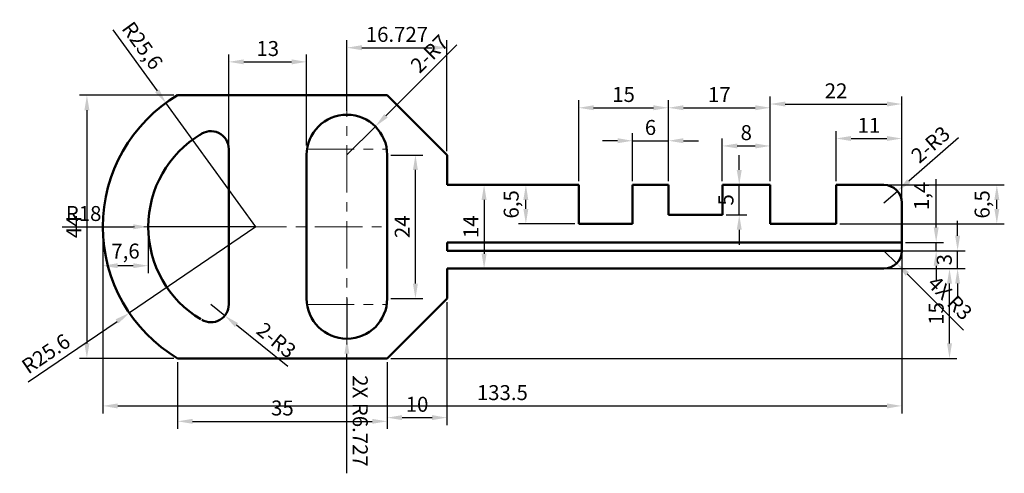
# Model space of a CAD drawing. Units: millimetres. Extents: x 2573 to 2737, y 1736 to 1812.
import ezdxf

# ---------------------------------------------------------------- set-up
doc = ezdxf.new("R2010")
doc.units = ezdxf.units.MM
doc.linetypes.add('CENTER', pattern=[50.8, 31.75, -6.35, 6.35, -6.35])
for name, color, linetype, lineweight in [('M-CNTR', 4, 'CENTER', 18), ('M-DIMS', 2, 'Continuous', 25), ('M-OUTL', 7, 'Continuous', 50)]:
    doc.layers.add(name, color=color, linetype=linetype, lineweight=lineweight)
doc.styles.get("Standard").update_dxf_attribs({"font": 'arial.ttf'})
doc.dimstyles.new('ISO-25', dxfattribs={"dimtxt": 2.5, "dimasz": 2.5, "dimexe": 1.25, "dimexo": 0.625, "dimtad": 1, "dimtxsty": 'Standard', "dimcen": 2.5, "dimadec": 0, "dimazin": 0, "dimtfac": 1, "dimtmove": 0, "dimatfit": 3, "dimfxl": 1, "dimarcsym": 0})

# ---------------------------------------------------------------- blocks, each defined once
blk = doc.blocks.new('*D1')
at = {"layer": 'Defpoints', "color": 0, "transparency": 16777216}
for p in [(2599.21, 1799.66), (2584.05, 1755.66), (2599.21, 1755.66)]:
    blk.add_point(p, dxfattribs=at)
at = {"layer": 'M-DIMS', "color": 0, "lineweight": -2, "transparency": 16777216}
for p, q in [((2598.59, 1799.66), (2582.8, 1799.66)), ((2584.05, 1797.16), (2584.05, 1758.16)), ((2598.59, 1755.66), (2582.8, 1755.66))]:
    blk.add_line(p, q, dxfattribs=at)
at = {"layer": 'M-DIMS', "color": 0, "transparency": 16777216}
for points in [[(2583.63, 1797.16), (2584.47, 1797.16), (2584.05, 1799.66)], [(2583.63, 1758.16), (2584.47, 1758.16), (2584.05, 1755.66)]]:
    blk.add_solid(points, dxfattribs=at)
at = {"layer": 'M-DIMS', "color": 0, "transparency": 16777216, "insert": (2582.17, 1777.66), "char_height": 2.5, "attachment_point": 5, "rotation": 90}
blk.add_mtext('44', dxfattribs=at)
blk = doc.blocks.new('*D2')
at = {"layer": 'Defpoints', "color": 0, "transparency": 16777216}
for p in [(2620.76, 1805.24), (2607.76, 1790.66), (2620.76, 1790.66)]:
    blk.add_point(p, dxfattribs=at)
at = {"layer": 'M-DIMS', "color": 0, "lineweight": -2, "transparency": 16777216}
for p, q in [((2607.76, 1791.28), (2607.76, 1806.49)), ((2620.76, 1791.28), (2620.76, 1806.49)), ((2610.26, 1805.24), (2618.26, 1805.24))]:
    blk.add_line(p, q, dxfattribs=at)
at = {"layer": 'M-DIMS', "color": 0, "transparency": 16777216}
for points in [[(2610.26, 1805.65), (2610.26, 1804.82), (2607.76, 1805.24)], [(2618.26, 1805.65), (2618.26, 1804.82), (2620.76, 1805.24)]]:
    blk.add_solid(points, dxfattribs=at)
at = {"layer": 'M-DIMS', "color": 0, "transparency": 16777216, "insert": (2614.26, 1807.14), "char_height": 2.5, "attachment_point": 5}
blk.add_mtext('13', dxfattribs=at)
blk = doc.blocks.new('*D3')
at = {"layer": 'Defpoints', "color": 0, "transparency": 16777216}
for p in [(2599.21, 1755.66), (2634.21, 1755.66), (2634.21, 1745.13)]:
    blk.add_point(p, dxfattribs=at)
at = {"layer": 'M-DIMS', "color": 0, "lineweight": -2, "transparency": 16777216}
for p, q in [((2599.21, 1755.04), (2599.21, 1743.88)), ((2634.21, 1755.04), (2634.21, 1743.88)), ((2601.71, 1745.13), (2631.71, 1745.13))]:
    blk.add_line(p, q, dxfattribs=at)
at = {"layer": 'M-DIMS', "color": 0, "transparency": 16777216}
for points in [[(2601.71, 1745.55), (2601.71, 1744.72), (2599.21, 1745.13)], [(2631.71, 1745.55), (2631.71, 1744.72), (2634.21, 1745.13)]]:
    blk.add_solid(points, dxfattribs=at)
at = {"layer": 'M-DIMS', "color": 0, "transparency": 16777216, "insert": (2616.71, 1747.04), "char_height": 2.5, "attachment_point": 5}
blk.add_mtext('35', dxfattribs=at)
blk = doc.blocks.new('*D4')
at = {"layer": 'Defpoints', "color": 0, "transparency": 16777216}
for p in [(2644.21, 1765.66), (2634.21, 1755.66), (2644.21, 1745.75)]:
    blk.add_point(p, dxfattribs=at)
at = {"layer": 'M-DIMS', "color": 0, "lineweight": -2, "transparency": 16777216}
for p, q in [((2644.21, 1765.04), (2644.21, 1744.5)), ((2634.21, 1755.04), (2634.21, 1744.5)), ((2636.71, 1745.75), (2641.71, 1745.75))]:
    blk.add_line(p, q, dxfattribs=at)
at = {"layer": 'M-DIMS', "color": 0, "transparency": 16777216}
for points in [[(2636.71, 1746.17), (2636.71, 1745.34), (2634.21, 1745.75)], [(2641.71, 1746.17), (2641.71, 1745.34), (2644.21, 1745.75)]]:
    blk.add_solid(points, dxfattribs=at)
at = {"layer": 'M-DIMS', "color": 0, "transparency": 16777216, "insert": (2639.21, 1747.66), "char_height": 2.5, "attachment_point": 5}
blk.add_mtext('10', dxfattribs=at)
blk = doc.blocks.new('*D5')
at = {"layer": 'Defpoints', "color": 0, "transparency": 16777216}
for p in [(2657.39, 1784.66), (2666.21, 1784.66), (2666.21, 1778.16)]:
    blk.add_point(p, dxfattribs=at)
at = {"layer": 'M-DIMS', "color": 0, "lineweight": -2, "transparency": 16777216}
for p, q in [((2665.59, 1784.66), (2656.14, 1784.66)), ((2657.39, 1780.66), (2657.39, 1782.16)), ((2665.59, 1778.16), (2656.14, 1778.16))]:
    blk.add_line(p, q, dxfattribs=at)
at = {"layer": 'M-DIMS', "color": 0, "transparency": 16777216}
for points in [[(2656.97, 1782.16), (2657.8, 1782.16), (2657.39, 1784.66)], [(2656.97, 1780.66), (2657.8, 1780.66), (2657.39, 1778.16)]]:
    blk.add_solid(points, dxfattribs=at)
at = {"layer": 'M-DIMS', "color": 0, "transparency": 16777216, "insert": (2655.26, 1781.41), "char_height": 2.5, "attachment_point": 5, "rotation": 90}
blk.add_mtext('6,5', dxfattribs=at)
blk = doc.blocks.new('*D6')
at = {"layer": 'Defpoints', "color": 0, "transparency": 16777216}
for p in [(2644.21, 1784.66), (2644.21, 1770.66), (2650.41, 1770.66)]:
    blk.add_point(p, dxfattribs=at)
at = {"layer": 'M-DIMS', "color": 0, "lineweight": -2, "transparency": 16777216}
for p, q in [((2644.84, 1784.66), (2651.66, 1784.66)), ((2650.41, 1782.16), (2650.41, 1773.16)), ((2644.84, 1770.66), (2651.66, 1770.66))]:
    blk.add_line(p, q, dxfattribs=at)
at = {"layer": 'M-DIMS', "color": 0, "transparency": 16777216}
for points in [[(2649.99, 1782.16), (2650.83, 1782.16), (2650.41, 1784.66)], [(2649.99, 1773.16), (2650.83, 1773.16), (2650.41, 1770.66)]]:
    blk.add_solid(points, dxfattribs=at)
at = {"layer": 'M-DIMS', "color": 0, "transparency": 16777216, "insert": (2648.53, 1777.66), "char_height": 2.5, "attachment_point": 5, "rotation": 90}
blk.add_mtext('14', dxfattribs=at)
blk = doc.blocks.new('*D7')
at = {"layer": 'Defpoints', "color": 0, "transparency": 16777216}
for p in [(2634.21, 1789.66), (2638.94, 1789.66), (2634.21, 1765.66)]:
    blk.add_point(p, dxfattribs=at)
at = {"layer": 'M-DIMS', "color": 0, "lineweight": -2, "transparency": 16777216}
for p, q in [((2634.84, 1789.66), (2640.19, 1789.66)), ((2638.94, 1768.16), (2638.94, 1787.16)), ((2634.84, 1765.66), (2640.19, 1765.66))]:
    blk.add_line(p, q, dxfattribs=at)
at = {"layer": 'M-DIMS', "color": 0, "transparency": 16777216}
for points in [[(2638.52, 1787.16), (2639.35, 1787.16), (2638.94, 1789.66)], [(2638.52, 1768.16), (2639.35, 1768.16), (2638.94, 1765.66)]]:
    blk.add_solid(points, dxfattribs=at)
at = {"layer": 'M-DIMS', "color": 0, "transparency": 16777216, "insert": (2637.06, 1777.66), "char_height": 2.5, "attachment_point": 5, "rotation": 90}
blk.add_mtext('24', dxfattribs=at)
blk = doc.blocks.new('*D8')
at = {"layer": 'Defpoints', "color": 0, "transparency": 16777216}
for p in [(2681.21, 1797.56), (2666.21, 1784.66), (2681.21, 1784.66)]:
    blk.add_point(p, dxfattribs=at)
at = {"layer": 'M-DIMS', "color": 0, "lineweight": -2, "transparency": 16777216}
for p, q in [((2666.21, 1785.29), (2666.21, 1798.81)), ((2681.21, 1785.29), (2681.21, 1798.81)), ((2668.71, 1797.56), (2678.71, 1797.56))]:
    blk.add_line(p, q, dxfattribs=at)
at = {"layer": 'M-DIMS', "color": 0, "transparency": 16777216}
for points in [[(2668.71, 1797.98), (2668.71, 1797.15), (2666.21, 1797.56)], [(2678.71, 1797.98), (2678.71, 1797.15), (2681.21, 1797.56)]]:
    blk.add_solid(points, dxfattribs=at)
at = {"layer": 'M-DIMS', "color": 0, "transparency": 16777216, "insert": (2673.71, 1799.46), "char_height": 2.5, "attachment_point": 5}
blk.add_mtext('15', dxfattribs=at)
blk = doc.blocks.new('*D9')
at = {"layer": 'Defpoints', "color": 0, "transparency": 16777216}
for p in [(2698.21, 1797.56), (2681.21, 1784.66), (2698.21, 1784.66)]:
    blk.add_point(p, dxfattribs=at)
at = {"layer": 'M-DIMS', "color": 0, "lineweight": -2, "transparency": 16777216}
for p, q in [((2681.21, 1785.29), (2681.21, 1798.81)), ((2698.21, 1785.29), (2698.21, 1798.81)), ((2683.71, 1797.56), (2695.71, 1797.56))]:
    blk.add_line(p, q, dxfattribs=at)
at = {"layer": 'M-DIMS', "color": 0, "transparency": 16777216}
for points in [[(2683.71, 1797.98), (2683.71, 1797.15), (2681.21, 1797.56)], [(2695.71, 1797.98), (2695.71, 1797.15), (2698.21, 1797.56)]]:
    blk.add_solid(points, dxfattribs=at)
at = {"layer": 'M-DIMS', "color": 0, "transparency": 16777216, "insert": (2689.71, 1799.44), "char_height": 2.5, "attachment_point": 5}
blk.add_mtext('17', dxfattribs=at)
blk = doc.blocks.new('*D10')
at = {"layer": 'Defpoints', "color": 0, "transparency": 16777216}
for p in [(2720.21, 1798.19), (2698.21, 1784.66), (2720.21, 1781.66)]:
    blk.add_point(p, dxfattribs=at)
at = {"layer": 'M-DIMS', "color": 0, "lineweight": -2, "transparency": 16777216}
for p, q in [((2698.21, 1785.29), (2698.21, 1799.44)), ((2700.71, 1798.19), (2717.71, 1798.19)), ((2720.21, 1782.29), (2720.21, 1799.44))]:
    blk.add_line(p, q, dxfattribs=at)
at = {"layer": 'M-DIMS', "color": 0, "transparency": 16777216}
for points in [[(2700.71, 1798.6), (2700.71, 1797.77), (2698.21, 1798.19)], [(2717.71, 1798.6), (2717.71, 1797.77), (2720.21, 1798.19)]]:
    blk.add_solid(points, dxfattribs=at)
at = {"layer": 'M-DIMS', "color": 0, "transparency": 16777216, "insert": (2709.21, 1800.07), "char_height": 2.5, "attachment_point": 5}
blk.add_mtext('22', dxfattribs=at)
blk = doc.blocks.new('*D11')
at = {"layer": 'Defpoints', "color": 0, "transparency": 16777216}
for p in [(2720.21, 1792.42), (2709.21, 1784.66), (2720.21, 1781.66)]:
    blk.add_point(p, dxfattribs=at)
at = {"layer": 'M-DIMS', "color": 0, "lineweight": -2, "transparency": 16777216}
for p, q in [((2709.21, 1785.29), (2709.21, 1793.67)), ((2720.21, 1782.29), (2720.21, 1793.67)), ((2711.71, 1792.42), (2717.71, 1792.42))]:
    blk.add_line(p, q, dxfattribs=at)
at = {"layer": 'M-DIMS', "color": 0, "transparency": 16777216}
for points in [[(2711.71, 1792.84), (2711.71, 1792.01), (2709.21, 1792.42)], [(2717.71, 1792.84), (2717.71, 1792.01), (2720.21, 1792.42)]]:
    blk.add_solid(points, dxfattribs=at)
at = {"layer": 'M-DIMS', "color": 0, "transparency": 16777216, "insert": (2714.71, 1794.3), "char_height": 2.5, "attachment_point": 5}
blk.add_mtext('11', dxfattribs=at)
blk = doc.blocks.new('*D12')
at = {"layer": 'Defpoints', "color": 0, "transparency": 16777216}
for p in [(2698.21, 1791.18), (2690.21, 1784.66), (2698.21, 1784.66)]:
    blk.add_point(p, dxfattribs=at)
at = {"layer": 'M-DIMS', "color": 0, "lineweight": -2, "transparency": 16777216}
for p, q in [((2690.21, 1785.29), (2690.21, 1792.43)), ((2698.21, 1785.29), (2698.21, 1792.43)), ((2692.71, 1791.18), (2695.71, 1791.18))]:
    blk.add_line(p, q, dxfattribs=at)
at = {"layer": 'M-DIMS', "color": 0, "transparency": 16777216}
for points in [[(2692.71, 1791.59), (2692.71, 1790.76), (2690.21, 1791.18)], [(2695.71, 1791.59), (2695.71, 1790.76), (2698.21, 1791.18)]]:
    blk.add_solid(points, dxfattribs=at)
at = {"layer": 'M-DIMS', "color": 0, "transparency": 16777216, "insert": (2694.21, 1793.08), "char_height": 2.5, "attachment_point": 5}
blk.add_mtext('8', dxfattribs=at)
blk = doc.blocks.new('*D13')
at = {"layer": 'Defpoints', "color": 0, "transparency": 16777216}
for p in [(2681.21, 1792.05), (2675.21, 1784.66), (2681.21, 1784.66)]:
    blk.add_point(p, dxfattribs=at)
at = {"layer": 'M-DIMS', "color": 0, "lineweight": -2, "transparency": 16777216}
for p, q in [((2675.21, 1785.29), (2675.21, 1793.3)), ((2681.21, 1785.29), (2681.21, 1793.3)), ((2672.71, 1792.05), (2670.21, 1792.05)), ((2675.21, 1792.05), (2681.21, 1792.05)), ((2683.71, 1792.05), (2686.21, 1792.05))]:
    blk.add_line(p, q, dxfattribs=at)
at = {"layer": 'M-DIMS', "color": 0, "transparency": 16777216}
for points in [[(2672.71, 1792.47), (2672.71, 1791.63), (2675.21, 1792.05)], [(2683.71, 1792.47), (2683.71, 1791.63), (2681.21, 1792.05)]]:
    blk.add_solid(points, dxfattribs=at)
at = {"layer": 'M-DIMS', "color": 0, "transparency": 16777216, "insert": (2678.21, 1793.95), "char_height": 2.5, "attachment_point": 5}
blk.add_mtext('6', dxfattribs=at)
blk = doc.blocks.new('*D14')
at = {"layer": 'Defpoints', "color": 0, "transparency": 16777216}
for p in [(2690.21, 1784.66), (2693.04, 1784.66), (2690.21, 1779.66)]:
    blk.add_point(p, dxfattribs=at)
at = {"layer": 'M-DIMS', "color": 0, "lineweight": -2, "transparency": 16777216}
for p, q in [((2693.04, 1787.16), (2693.04, 1789.66)), ((2690.84, 1784.66), (2694.29, 1784.66)), ((2693.04, 1779.66), (2693.04, 1784.66)), ((2690.84, 1779.66), (2694.29, 1779.66)), ((2693.04, 1777.16), (2693.04, 1774.66))]:
    blk.add_line(p, q, dxfattribs=at)
at = {"layer": 'M-DIMS', "color": 0, "transparency": 16777216}
for points in [[(2692.62, 1787.16), (2693.45, 1787.16), (2693.04, 1784.66)], [(2692.62, 1777.16), (2693.45, 1777.16), (2693.04, 1779.66)]]:
    blk.add_solid(points, dxfattribs=at)
at = {"layer": 'M-DIMS', "color": 0, "transparency": 16777216, "insert": (2691.14, 1782.16), "char_height": 2.5, "attachment_point": 5, "rotation": 90}
blk.add_mtext('5', dxfattribs=at)
blk = doc.blocks.new('*D15')
at = {"layer": 'Defpoints', "color": 0, "transparency": 16777216}
for p in [(2720.21, 1775.06), (2725.94, 1775.06), (2720.21, 1773.66)]:
    blk.add_point(p, dxfattribs=at)
at = {"layer": 'M-DIMS', "color": 0, "lineweight": -2, "transparency": 16777216}
for p, q in [((2725.94, 1777.56), (2725.94, 1785.62)), ((2720.84, 1775.06), (2727.19, 1775.06)), ((2725.94, 1773.66), (2725.94, 1775.06)), ((2720.84, 1773.66), (2727.19, 1773.66)), ((2725.94, 1771.16), (2725.94, 1768.66))]:
    blk.add_line(p, q, dxfattribs=at)
at = {"layer": 'M-DIMS', "color": 0, "transparency": 16777216}
for points in [[(2725.52, 1777.56), (2726.35, 1777.56), (2725.94, 1775.06)], [(2725.52, 1771.16), (2726.35, 1771.16), (2725.94, 1773.66)]]:
    blk.add_solid(points, dxfattribs=at)
at = {"layer": 'M-DIMS', "color": 0, "transparency": 16777216, "insert": (2723.81, 1782.84), "char_height": 2.5, "attachment_point": 5, "rotation": 90}
blk.add_mtext('1,4', dxfattribs=at)
blk = doc.blocks.new('*D16')
at = {"layer": 'Defpoints', "color": 0, "transparency": 16777216}
for p in [(2717.21, 1773.66), (2729.52, 1773.66), (2717.21, 1770.66)]:
    blk.add_point(p, dxfattribs=at)
at = {"layer": 'M-DIMS', "color": 0, "lineweight": -2, "transparency": 16777216}
for p, q in [((2729.52, 1776.16), (2729.52, 1778.66)), ((2717.84, 1773.66), (2730.77, 1773.66)), ((2729.52, 1770.66), (2729.52, 1773.66)), ((2717.84, 1770.66), (2730.77, 1770.66)), ((2729.52, 1768.16), (2729.52, 1765.66))]:
    blk.add_line(p, q, dxfattribs=at)
at = {"layer": 'M-DIMS', "color": 0, "transparency": 16777216}
for points in [[(2729.11, 1776.16), (2729.94, 1776.16), (2729.52, 1773.66)], [(2729.11, 1768.16), (2729.94, 1768.16), (2729.52, 1770.66)]]:
    blk.add_solid(points, dxfattribs=at)
at = {"layer": 'M-DIMS', "color": 0, "transparency": 16777216, "insert": (2727.62, 1772.16), "char_height": 2.5, "attachment_point": 5, "rotation": 90}
blk.add_mtext('3', dxfattribs=at)
blk = doc.blocks.new('*D17')
at = {"layer": 'Defpoints', "color": 0, "transparency": 16777216}
for p in [(2709.21, 1784.66), (2736.07, 1784.66), (2709.21, 1778.16)]:
    blk.add_point(p, dxfattribs=at)
at = {"layer": 'M-DIMS', "color": 0, "lineweight": -2, "transparency": 16777216}
for p, q in [((2709.84, 1784.66), (2737.32, 1784.66)), ((2736.07, 1780.66), (2736.07, 1782.16)), ((2709.84, 1778.16), (2737.32, 1778.16))]:
    blk.add_line(p, q, dxfattribs=at)
at = {"layer": 'M-DIMS', "color": 0, "transparency": 16777216}
for points in [[(2735.66, 1782.16), (2736.49, 1782.16), (2736.07, 1784.66)], [(2735.66, 1780.66), (2736.49, 1780.66), (2736.07, 1778.16)]]:
    blk.add_solid(points, dxfattribs=at)
at = {"layer": 'M-DIMS', "color": 0, "transparency": 16777216, "insert": (2733.94, 1781.41), "char_height": 2.5, "attachment_point": 5, "rotation": 90}
blk.add_mtext('6,5', dxfattribs=at)
blk = doc.blocks.new('*D18')
at = {"layer": 'Defpoints', "color": 0, "transparency": 16777216}
for p in [(2586.7, 1777.66), (2594.3, 1777.66), (2586.7, 1771.16)]:
    blk.add_point(p, dxfattribs=at)
at = {"layer": 'M-DIMS', "color": 0, "lineweight": -2, "transparency": 16777216}
for p, q in [((2586.7, 1777.04), (2586.7, 1769.91)), ((2594.3, 1777.04), (2594.3, 1769.91)), ((2591.8, 1771.16), (2589.2, 1771.16))]:
    blk.add_line(p, q, dxfattribs=at)
at = {"layer": 'M-DIMS', "color": 0, "transparency": 16777216}
for points in [[(2589.2, 1771.57), (2589.2, 1770.74), (2586.7, 1771.16)], [(2591.8, 1771.57), (2591.8, 1770.74), (2594.3, 1771.16)]]:
    blk.add_solid(points, dxfattribs=at)
at = {"layer": 'M-DIMS', "color": 0, "transparency": 16777216, "insert": (2590.5, 1773.28), "char_height": 2.5, "attachment_point": 5}
blk.add_mtext('7,6', dxfattribs=at)
blk = doc.blocks.new('*D19')
at = {"layer": 'Defpoints', "color": 0, "transparency": 16777216}
for p in [(2597.26, 1798.37), (2612.3, 1777.66)]:
    blk.add_point(p, dxfattribs=at)
at = {"layer": 'M-DIMS', "color": 0, "lineweight": -2, "transparency": 16777216}
for p, q in [((2588.37, 1810.62), (2595.79, 1800.4)), ((2612.3, 1777.66), (2597.26, 1798.37))]:
    blk.add_line(p, q, dxfattribs=at)
at = {"layer": 'M-DIMS', "color": 0, "transparency": 16777216}
blk.add_solid([(2596.13, 1800.64), (2595.45, 1800.15), (2597.26, 1798.37)], dxfattribs=at)
at = {"layer": 'M-DIMS', "color": 0, "transparency": 16777216, "insert": (2593.07, 1807.77), "char_height": 2.5, "attachment_point": 5, "rotation": 305.9889}
blk.add_mtext('R25,6', dxfattribs=at)
blk = doc.blocks.new('*D20')
at = {"layer": 'Defpoints', "color": 0, "transparency": 16777216}
for p in [(2604.76, 1764.7), (2607.09, 1762.81)]:
    blk.add_point(p, dxfattribs=at)
at = {"layer": 'M-DIMS', "color": 0, "lineweight": -2, "transparency": 16777216}
for p, q in [((2604.76, 1764.7), (2607.09, 1762.81)), ((2617.64, 1754.28), (2609.04, 1761.24))]:
    blk.add_line(p, q, dxfattribs=at)
at = {"layer": 'M-DIMS', "color": 0, "transparency": 16777216}
blk.add_solid([(2609.3, 1761.56), (2608.77, 1760.91), (2607.09, 1762.81)], dxfattribs=at)
at = {"layer": 'M-DIMS', "color": 0, "transparency": 16777216, "insert": (2615.5, 1758.45), "char_height": 2.5, "attachment_point": 5, "rotation": 321.0342}
blk.add_mtext('2-R3', dxfattribs=at)
blk = doc.blocks.new('*D21')
at = {"layer": 'Defpoints', "color": 0, "transparency": 16777216}
for p in [(2632.24, 1794.44), (2627.49, 1789.68)]:
    blk.add_point(p, dxfattribs=at)
at = {"layer": 'M-DIMS', "color": 0, "lineweight": -2, "transparency": 16777216}
for p, q in [((2645.85, 1808.07), (2634.01, 1796.21)), ((2627.49, 1789.68), (2632.24, 1794.44))]:
    blk.add_line(p, q, dxfattribs=at)
at = {"layer": 'M-DIMS', "color": 0, "transparency": 16777216}
blk.add_solid([(2633.71, 1796.5), (2634.3, 1795.91), (2632.24, 1794.44)], dxfattribs=at)
at = {"layer": 'M-DIMS', "color": 0, "transparency": 16777216, "insert": (2641.5, 1806.37), "char_height": 2.5, "attachment_point": 5, "rotation": 45.0456}
blk.add_mtext('2-R7', dxfattribs=at)
blk = doc.blocks.new('*D22')
at = {"layer": 'Defpoints', "color": 0, "transparency": 16777216}
for p in [(2719.47, 1783.64), (2717.21, 1781.66)]:
    blk.add_point(p, dxfattribs=at)
at = {"layer": 'M-DIMS', "color": 0, "lineweight": -2, "transparency": 16777216}
for p, q in [((2729.68, 1792.56), (2721.35, 1785.28)), ((2717.21, 1781.66), (2719.47, 1783.64))]:
    blk.add_line(p, q, dxfattribs=at)
at = {"layer": 'M-DIMS', "color": 0, "transparency": 16777216}
blk.add_solid([(2721.08, 1785.59), (2721.63, 1784.97), (2719.47, 1783.64)], dxfattribs=at)
at = {"layer": 'M-DIMS', "color": 0, "transparency": 16777216, "insert": (2725.21, 1791.18), "char_height": 2.5, "attachment_point": 5, "rotation": 41.1657}
blk.add_mtext('2-R3', dxfattribs=at)
blk = doc.blocks.new('*D23')
at = {"layer": 'Defpoints', "color": 0, "transparency": 16777216}
for p in [(2720.21, 1781.66), (2586.7, 1777.66), (2720.21, 1747.71)]:
    blk.add_point(p, dxfattribs=at)
at = {"layer": 'M-DIMS', "color": 0, "lineweight": -2, "transparency": 16777216}
for p, q in [((2720.21, 1781.04), (2720.21, 1746.46)), ((2586.7, 1777.04), (2586.7, 1746.46)), ((2589.2, 1747.71), (2717.71, 1747.71))]:
    blk.add_line(p, q, dxfattribs=at)
at = {"layer": 'M-DIMS', "color": 0, "transparency": 16777216}
for points in [[(2589.2, 1748.13), (2589.2, 1747.29), (2586.7, 1747.71)], [(2717.71, 1748.13), (2717.71, 1747.29), (2720.21, 1747.71)]]:
    blk.add_solid(points, dxfattribs=at)
at = {"layer": 'M-DIMS', "color": 0, "transparency": 16777216, "insert": (2653.46, 1749.61), "char_height": 2.5, "attachment_point": 5}
blk.add_mtext('133.5', dxfattribs=at)
blk = doc.blocks.new('*D24')
at = {"layer": 'Defpoints', "color": 0, "transparency": 16777216}
for p in [(2644.21, 1807.61), (2627.49, 1796.4), (2644.21, 1789.66)]:
    blk.add_point(p, dxfattribs=at)
at = {"layer": 'M-DIMS', "color": 0, "lineweight": -2, "transparency": 16777216}
for p, q in [((2627.49, 1797.03), (2627.49, 1808.86)), ((2644.21, 1790.29), (2644.21, 1808.86)), ((2629.99, 1807.61), (2641.71, 1807.61))]:
    blk.add_line(p, q, dxfattribs=at)
at = {"layer": 'M-DIMS', "color": 0, "transparency": 16777216}
for points in [[(2629.99, 1808.03), (2629.99, 1807.19), (2627.49, 1807.61)], [(2641.71, 1808.03), (2641.71, 1807.19), (2644.21, 1807.61)]]:
    blk.add_solid(points, dxfattribs=at)
at = {"layer": 'M-DIMS', "color": 0, "transparency": 16777216, "insert": (2635.85, 1809.51), "char_height": 2.5, "attachment_point": 5}
blk.add_mtext('16.727', dxfattribs=at)
blk = doc.blocks.new('*D25')
at = {"layer": 'Defpoints', "color": 0, "transparency": 16777216}
for p in [(2644.21, 1770.66), (2728.16, 1770.66), (2634.21, 1755.66)]:
    blk.add_point(p, dxfattribs=at)
at = {"layer": 'M-DIMS', "color": 0, "lineweight": -2, "transparency": 16777216}
for p, q in [((2644.84, 1770.66), (2729.41, 1770.66)), ((2728.16, 1758.16), (2728.16, 1768.16)), ((2634.84, 1755.66), (2729.41, 1755.66))]:
    blk.add_line(p, q, dxfattribs=at)
at = {"layer": 'M-DIMS', "color": 0, "transparency": 16777216}
for points in [[(2727.75, 1768.16), (2728.58, 1768.16), (2728.16, 1770.66)], [(2727.75, 1758.16), (2728.58, 1758.16), (2728.16, 1755.66)]]:
    blk.add_solid(points, dxfattribs=at)
at = {"layer": 'M-DIMS', "color": 0, "transparency": 16777216, "insert": (2726.26, 1763.16), "char_height": 2.5, "attachment_point": 5, "rotation": 90}
blk.add_mtext('15', dxfattribs=at)
blk = doc.blocks.new('*D26')
at = {"layer": 'Defpoints', "color": 0, "transparency": 16777216}
for p in [(2612.3, 1777.66), (2591.14, 1763.25)]:
    blk.add_point(p, dxfattribs=at)
at = {"layer": 'M-DIMS', "color": 0, "lineweight": -2, "transparency": 16777216}
for p, q in [((2612.3, 1777.66), (2591.14, 1763.25)), ((2574.26, 1751.75), (2589.08, 1761.84))]:
    blk.add_line(p, q, dxfattribs=at)
at = {"layer": 'M-DIMS', "color": 0, "transparency": 16777216}
blk.add_solid([(2588.84, 1762.19), (2589.31, 1761.5), (2591.14, 1763.25)], dxfattribs=at)
at = {"layer": 'M-DIMS', "color": 0, "transparency": 16777216, "insert": (2577.38, 1756.18), "char_height": 2.5, "attachment_point": 5, "rotation": 34.2554}
blk.add_mtext('R25.6', dxfattribs=at)
blk = doc.blocks.new('*D27')
at = {"layer": 'Defpoints', "color": 0, "transparency": 16777216}
for p in [(2594.3, 1777.66), (2612.3, 1777.66)]:
    blk.add_point(p, dxfattribs=at)
at = {"layer": 'M-DIMS', "color": 0, "lineweight": -2, "transparency": 16777216}
for p, q in [((2579.89, 1777.66), (2591.8, 1777.66)), ((2612.3, 1777.66), (2594.3, 1777.66))]:
    blk.add_line(p, q, dxfattribs=at)
at = {"layer": 'M-DIMS', "color": 0, "transparency": 16777216}
blk.add_solid([(2591.8, 1778.08), (2591.8, 1777.24), (2594.3, 1777.66)], dxfattribs=at)
at = {"layer": 'M-DIMS', "color": 0, "transparency": 16777216, "insert": (2583.5, 1779.56), "char_height": 2.5, "attachment_point": 5, "rotation": 359.9993}
blk.add_mtext('R18', dxfattribs=at)
blk = doc.blocks.new('*D28')
at = {"layer": 'Defpoints', "color": 0, "transparency": 16777216}
for p in [(2627.49, 1765.66), (2627.49, 1758.93)]:
    blk.add_point(p, dxfattribs=at)
at = {"layer": 'M-DIMS', "color": 0, "lineweight": -2, "transparency": 16777216}
for p, q in [((2627.49, 1765.66), (2627.49, 1758.93)), ((2627.49, 1736.44), (2627.49, 1756.43))]:
    blk.add_line(p, q, dxfattribs=at)
at = {"layer": 'M-DIMS', "color": 0, "transparency": 16777216}
blk.add_solid([(2627.9, 1756.43), (2627.07, 1756.43), (2627.49, 1758.93)], dxfattribs=at)
at = {"layer": 'M-DIMS', "color": 0, "transparency": 16777216, "insert": (2629.39, 1745.19), "char_height": 2.5, "attachment_point": 5, "rotation": 270.0025}
blk.add_mtext('2X R6.727', dxfattribs=at)
blk = doc.blocks.new('*D29')
at = {"layer": 'Defpoints', "color": 0, "transparency": 16777216}
for p in [(2717.21, 1773.66), (2719.34, 1771.54)]:
    blk.add_point(p, dxfattribs=at)
at = {"layer": 'M-DIMS', "color": 0, "lineweight": -2, "transparency": 16777216}
for p, q in [((2717.21, 1773.66), (2719.34, 1771.54)), ((2730.48, 1760.4), (2721.1, 1769.77))]:
    blk.add_line(p, q, dxfattribs=at)
at = {"layer": 'M-DIMS', "color": 0, "transparency": 16777216}
blk.add_solid([(2721.4, 1770.07), (2720.81, 1769.48), (2719.34, 1771.54)], dxfattribs=at)
at = {"layer": 'M-DIMS', "color": 0, "transparency": 16777216, "insert": (2728.02, 1765.55), "char_height": 2.5, "attachment_point": 5, "rotation": 315.0122}
blk.add_mtext('4X R3', dxfattribs=at)

msp = doc.modelspace()

# ---------------------------------------------------------------- linework, layer by layer
at = {"layer": 'M-CNTR', "ltscale": 0.25, "transparency": 33554534}
for p, q in [((2627.4867, 1757.9691), (2627.4867, 1797.383)), ((2620.7601, 1790.6564), (2634.2133, 1790.6564)), ((2584.0484, 1777.6608), (2634.2133, 1777.6608)), ((2620.7601, 1764.6957), (2634.2133, 1764.6957))]:
    msp.add_line(p, q, dxfattribs=at)
at = {"layer": 'M-OUTL'}
for p, q in [((2599.2133, 1799.6608), (2634.2133, 1799.6608)), ((2644.2133, 1789.6608), (2634.2133, 1799.6608)), ((2607.7601, 1790.6564), (2607.7601, 1764.6957)), ((2620.7601, 1777.6761), (2620.7601, 1789.6761)), ((2634.2133, 1777.6608), (2634.2133, 1789.6608)), ((2644.2133, 1784.6608), (2644.2133, 1789.6608)), ((2666.2133, 1784.6608), (2644.2133, 1784.6608)), ((2666.2133, 1778.1608), (2666.2133, 1784.6608)), ((2681.2133, 1784.6608), (2675.2133, 1784.6608)), ((2675.2133, 1784.6608), (2675.2133, 1778.1608)), ((2681.2133, 1779.6608), (2681.2133, 1784.6608)), ((2698.2133, 1784.6608), (2690.2133, 1784.6608)), ((2690.2133, 1784.6608), (2690.2133, 1779.6608)), ((2698.2133, 1778.1608), (2698.2133, 1784.6608)), ((2709.2133, 1784.6608), (2717.2133, 1784.6608)), ((2709.2133, 1784.6608), (2709.2133, 1778.1608)), ((2720.2133, 1773.6608), (2720.2133, 1781.6608)), ((2690.2133, 1779.6608), (2681.2133, 1779.6608)), ((2620.7601, 1777.6761), (2620.7601, 1765.6761)), ((2634.2133, 1777.6608), (2634.2133, 1765.6608)), ((2675.2133, 1778.1608), (2666.2133, 1778.1608)), ((2709.2133, 1778.1608), (2698.2133, 1778.1608)), ((2644.2133, 1775.0608), (2720.2133, 1775.0608)), ((2644.2133, 1773.6608), (2644.2133, 1775.0608)), ((2644.2133, 1773.6608), (2720.2133, 1773.6608)), ((2644.2133, 1770.6608), (2717.2133, 1770.6608)), ((2644.2133, 1765.6608), (2644.2133, 1770.6608)), ((2644.2133, 1765.6608), (2634.2133, 1755.6608)), ((2634.2133, 1755.6608), (2599.2133, 1755.6608))]:
    msp.add_line(p, q, dxfattribs=at)
for centre, radius, start, end in [((2612.3038, 1777.6608), 25.6, 120.75352, 239.24648), ((2627.4867, 1789.6761), 6.7266, 0, 180), ((2612.3038, 1777.6608), 18, 120.75352, 239.24648), ((2604.7601, 1790.6564), 3, 0, 128.474033), ((2717.2133, 1781.6608), 3, 0, 90), ((2717.2133, 1773.6608), 3, 270, 0), ((2627.4867, 1765.6608), 6.7266, 180, 0), ((2604.7601, 1764.6957), 3, 239.806989, 0)]:
    msp.add_arc(centre, radius, start, end, dxfattribs=at)

# ---------------------------------------------------------------- dimensions: what is measured, and where the dimension line sits
at = {"layer": 'M-DIMS'}
dim = msp.add_radius_dim(center=(2612.3038, 1777.6608), mpoint=(2597.2605, 1798.3745), dimstyle='ISO-25', override={"dimclrd": 0, "dimclre": 0, "dimclrt": 0}, dxfattribs=at)
dim.commit()
dim.dimension.update_dxf_attribs({"geometry": '*D19', "text_midpoint": (2593.066, 1807.7704)})
for base, p1, p2, override, picture, middle in [((2644.2133, 1807.6108), (2627.4867, 1796.4027), (2644.2133, 1789.6608), {"dimdec": 3, "dimlfac": 1, "dimrnd": 0, "dimzin": 0, "dimdsep": 46, "dimlunit": 2}, '*D24', (2635.85, 1809.5122)), ((2620.7601, 1805.2353), (2607.7601, 1790.6564), (2620.7601, 1790.6564), {"dimclrd": 0, "dimclre": 0, "dimclrt": 0}, '*D2', (2614.2601, 1807.1376)), ((2720.2133, 1798.1864), (2698.2133, 1784.6608), (2720.2133, 1781.6608), {"dimclrd": 0, "dimclre": 0, "dimclrt": 0}, '*D10', (2709.2133, 1800.0665)), ((2681.2133, 1797.5632), (2666.2133, 1784.6608), (2681.2133, 1784.6608), {"dimclrd": 0, "dimclre": 0, "dimclrt": 0}, '*D8', (2673.7133, 1799.4647)), ((2698.2133, 1797.5632), (2681.2133, 1784.6608), (2698.2133, 1784.6608), {"dimclrd": 0, "dimclre": 0, "dimclrt": 0}, '*D9', (2689.7133, 1799.4434)), ((2681.2133, 1792.0495), (2675.2133, 1784.6608), (2681.2133, 1784.6608), {"dimclrd": 0, "dimclre": 0, "dimclrt": 0}, '*D13', (2678.2133, 1793.9509)), ((2698.2133, 1791.1763), (2690.2133, 1784.6608), (2698.2133, 1784.6608), {"dimclrd": 0, "dimclre": 0, "dimclrt": 0}, '*D12', (2694.2133, 1793.0777)), ((2720.2133, 1792.4225), (2709.2133, 1784.6608), (2720.2133, 1781.6608), {"dimclrd": 0, "dimclre": 0, "dimclrt": 0}, '*D11', (2714.7133, 1794.3027)), ((2720.2133, 1747.7108), (2586.7038, 1777.6608), (2720.2133, 1781.6608), {"dimdec": 1, "dimlfac": 1, "dimrnd": 0, "dimzin": 0, "dimdsep": 46, "dimlunit": 2}, '*D23', (2653.4586, 1749.6131)), ((2644.2133, 1745.7538), (2634.2133, 1755.6608), (2644.2133, 1765.6608), {"dimclrd": 0, "dimclre": 0, "dimclrt": 0}, '*D4', (2639.2133, 1747.6552)), ((2634.2133, 1745.1342), (2599.2133, 1755.6608), (2634.2133, 1755.6608), {"dimclrd": 0, "dimclre": 0, "dimclrt": 0}, '*D3', (2616.7133, 1747.0365))]:
    dim = msp.add_linear_dim(base=base, p1=p1, p2=p2, dimstyle='ISO-25', override=override, dxfattribs=at)
    dim.commit()
    dim.dimension.update_dxf_attribs({"geometry": picture, "text_midpoint": middle})
dim = msp.add_radius_dim(center=(2627.4867, 1789.6761), mpoint=(2632.2394, 1794.4363), text='2-<>', dimstyle='ISO-25', override={"dimdec": 0, "dimclrd": 0, "dimclre": 0, "dimclrt": 0}, dxfattribs=at)
dim.commit()
dim.dimension.update_dxf_attribs({"geometry": '*D21', "text_midpoint": (2642.8268, 1805.0406), "dimtype": 164})
for base, p1, p2, override, picture, middle in [((2584.0484, 1755.6608), (2599.2133, 1799.6608), (2599.2133, 1755.6608), {"dimclrd": 0, "dimclre": 0, "dimclrt": 0}, '*D1', (2582.1734, 1777.6608)), ((2638.9379, 1789.6608), (2634.2133, 1765.6608), (2634.2133, 1789.6608), {"dimclrd": 0, "dimclre": 0, "dimclrt": 0}, '*D7', (2637.0578, 1777.6608)), ((2693.0356, 1784.6608), (2690.2133, 1779.6608), (2690.2133, 1784.6608), {"dimclrd": 0, "dimclre": 0, "dimclrt": 0}, '*D14', (2691.1393, 1782.1608)), ((2725.9364, 1775.0608), (2720.2133, 1773.6608), (2720.2133, 1775.0608), {"dimclrd": 0, "dimclre": 0, "dimclrt": 0}, '*D15', (2723.809, 1782.8387)), ((2650.409, 1770.6608), (2644.2133, 1784.6608), (2644.2133, 1770.6608), {"dimclrd": 0, "dimclre": 0, "dimclrt": 0}, '*D6', (2648.5289, 1777.6608)), ((2657.3862, 1784.6608), (2666.2133, 1778.1608), (2666.2133, 1784.6608), {"dimclrd": 0, "dimclre": 0, "dimclrt": 0}, '*D5', (2655.2588, 1781.4108)), ((2736.0718, 1784.6608), (2709.2133, 1778.1608), (2709.2133, 1784.6608), {"dimclrd": 0, "dimclre": 0, "dimclrt": 0}, '*D17', (2733.9444, 1781.4108)), ((2729.5228, 1773.6608), (2717.2133, 1770.6608), (2717.2133, 1773.6608), {"dimclrd": 0, "dimclre": 0, "dimclrt": 0}, '*D16', (2727.6205, 1772.1608)), ((2728.1633, 1770.6608), (2634.2133, 1755.6608), (2644.2133, 1770.6608), {"dimdec": 0, "dimlfac": 1, "dimrnd": 0, "dimzin": 0, "dimdsep": 46, "dimlunit": 2}, '*D25', (2726.2619, 1763.1608))]:
    dim = msp.add_linear_dim(base=base, p1=p1, p2=p2, angle=90, dimstyle='ISO-25', override=override, dxfattribs=at)
    dim.commit()
    dim.dimension.update_dxf_attribs({"geometry": picture, "text_midpoint": middle})
for center, mpoint, text, override, picture, middle in [((2717.2133, 1781.6608), (2719.4718, 1783.6355), '2-<>', {"dimclrd": 0, "dimclre": 0, "dimclrt": 0}, '*D22', (2725.2053, 1791.1757)), ((2717.2133, 1773.6608), (2719.3351, 1771.5399), '4X <>', {"dimdec": 0, "dimlfac": 1, "dimrnd": 0, "dimzin": 0, "dimdsep": 46, "dimlunit": 2}, '*D29', (2728.0191, 1765.5493)), ((2627.4867, 1765.6608), (2627.487, 1758.9341), '2X <>', {"dimdec": 3, "dimlfac": 1, "dimrnd": 0, "dimzin": 0, "dimdsep": 46, "dimlunit": 2}, '*D28', (2629.389, 1745.1876)), ((2604.7601, 1764.6957), (2607.0926, 1762.8092), '2-<>', {"dimclrd": 0, "dimclre": 0, "dimclrt": 0}, '*D20', (2615.5039, 1758.4527))]:
    dim = msp.add_radius_dim(center=center, mpoint=mpoint, text=text, dimstyle='ISO-25', override=override, dxfattribs=at)
    dim.commit()
    dim.dimension.update_dxf_attribs({"geometry": picture, "text_midpoint": middle})
for mpoint, override, picture, middle in [((2594.3038, 1777.661), {"dimdec": 0, "dimlfac": 1, "dimrnd": 0, "dimzin": 0, "dimdsep": 46, "dimlunit": 2}, '*D27', (2583.5038, 1777.6611)), ((2591.1444, 1763.251), {"dimdec": 1, "dimlfac": 1, "dimrnd": 0, "dimzin": 0, "dimdsep": 46, "dimlunit": 2}, '*D26', (2578.4488, 1754.6051))]:
    dim = msp.add_radius_dim(center=(2612.3038, 1777.6608), mpoint=mpoint, dimstyle='ISO-25', override=override, dxfattribs=at)
    dim.commit()
    dim.dimension.update_dxf_attribs({"geometry": picture, "text_midpoint": middle, "dimtype": 164})
dim = msp.add_aligned_dim(p1=(2594.3038, 1777.6608), p2=(2586.7038, 1777.6608), distance=6.5034, dimstyle='ISO-25', override={"dimclrd": 0, "dimclre": 0, "dimclrt": 0}, dxfattribs=at)
dim.commit()
dim.dimension.update_dxf_attribs({"geometry": '*D18', "text_midpoint": (2590.5038, 1773.2847)})

doc.saveas('drawing.dxf')
